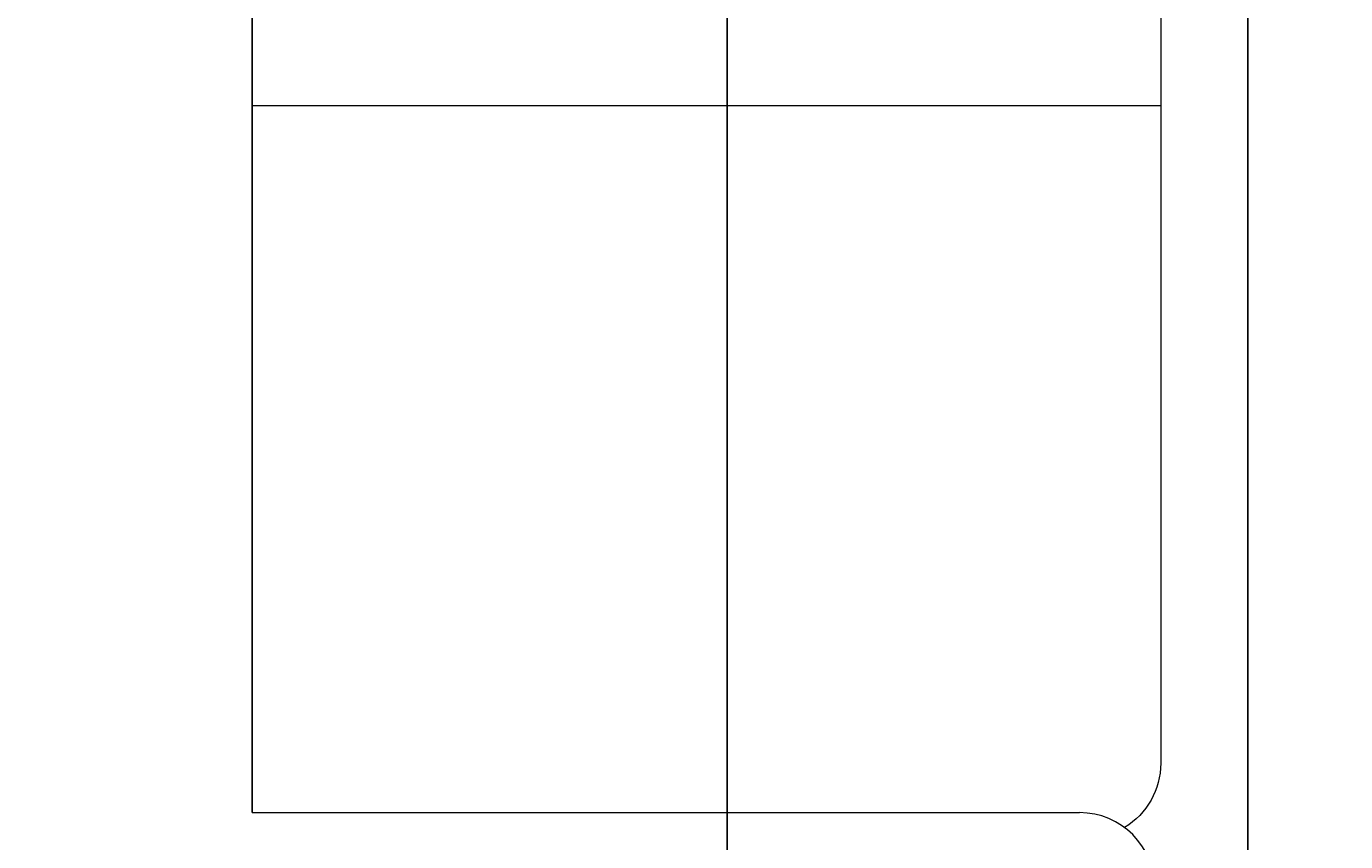
# Model space of a CAD drawing. Units: inches. Extents: x 2231 to 2461, y 2045 to 2455.
# Tile 39 of 95: x 2262 to 2297, y 2200 to 2222. Entities that reach past the tile are written whole.
import ezdxf

# ---------------------------------------------------------------- set-up
doc = ezdxf.new("R2010")
doc.units = ezdxf.units.IN
doc.layers.add('A-ANNO-DIMS', color=2, linetype='Continuous', lineweight=18)
doc.layers.add('A-FURN', color=9, linetype='Continuous', lineweight=18)
doc.styles.get("Standard").update_dxf_attribs({"font": 'arial.ttf'})
doc.dimstyles.get("Standard").update_dxf_attribs({"dimtxt": 0.18, "dimasz": 0.18, "dimexe": 0.18, "dimexo": 0.0625, "dimgap": 0.09, "dimtad": 0, "dimtih": 1, "dimtoh": 1, "dimdec": 4, "dimzin": 0, "dimdsep": 46, "dimtxsty": 'Standard', "dimcen": 0.09, "dimadec": 0, "dimazin": 0, "dimtfac": 1, "dimtdec": 4, "dimtofl": 0, "dimtmove": 0, "dimatfit": 3, "dimfxl": 1, "dimtolj": 1, "dimtzin": 0, "dimarcsym": 0})

# ---------------------------------------------------------------- blocks, each defined once
blk = doc.blocks.new('*D47')
at = {"layer": 'A-ANNO-DIMS', "color": 0, "lineweight": -2, "transparency": 16777216}
for p, q in [((2258.794, 2182.895), (2258.794, 2454.645)), ((2258.974, 2454.465), (2276.575, 2454.465)), ((2294.614, 2454.465), (2277.012, 2454.465)), ((2294.794, 2182.895), (2294.794, 2454.645))]:
    blk.add_line(p, q, dxfattribs=at)
at = {"layer": 'A-ANNO-DIMS', "color": 0, "transparency": 16777216}
for points in [[(2258.974, 2454.495), (2258.974, 2454.435), (2258.794, 2454.465)], [(2294.614, 2454.495), (2294.614, 2454.435), (2294.794, 2454.465)]]:
    blk.add_solid(points, dxfattribs=at)
at = {"layer": 'Defpoints', "color": 0, "transparency": 16777216}
for p in [(2294.794, 2454.465), (2258.794, 2182.833), (2294.794, 2182.833)]:
    blk.add_point(p, dxfattribs=at)
at = {"layer": 'A-ANNO-DIMS', "color": 0, "transparency": 16777216, "insert": (2276.794, 2454.465), "char_height": 0.18, "attachment_point": 5}
blk.add_mtext('\\A1;36', dxfattribs=at)
blk = doc.blocks.new('*D51')
at = {"layer": 'A-ANNO-DIMS', "color": 0, "lineweight": -2, "transparency": 16777216}
for p, q in [((2258.794, 2306.77), (2258.794, 2044.803)), ((2330.794, 2306.77), (2330.794, 2044.803)), ((2258.974, 2044.983), (2294.576, 2044.983)), ((2330.614, 2044.983), (2295.011, 2044.983))]:
    blk.add_line(p, q, dxfattribs=at)
at = {"layer": 'A-ANNO-DIMS', "color": 0, "transparency": 16777216}
for points in [[(2258.974, 2045.013), (2258.974, 2044.953), (2258.794, 2044.983)], [(2330.614, 2045.013), (2330.614, 2044.953), (2330.794, 2044.983)]]:
    blk.add_solid(points, dxfattribs=at)
at = {"layer": 'Defpoints', "color": 0, "transparency": 16777216}
for p in [(2258.794, 2306.833), (2330.794, 2306.833), (2330.794, 2044.983)]:
    blk.add_point(p, dxfattribs=at)
at = {"layer": 'A-ANNO-DIMS', "color": 0, "transparency": 16777216, "insert": (2294.794, 2044.983), "char_height": 0.18, "attachment_point": 5}
blk.add_mtext('\\A1;72', dxfattribs=at)
blk = doc.blocks.new('*D63')
at = {"layer": 'A-ANNO-DIMS', "color": 0, "lineweight": -2, "transparency": 16777216}
for p, q in [((2262.383, 2255.114), (2281.133, 2255.114)), ((2280.953, 2254.934), (2280.953, 2225.296)), ((2280.953, 2195.294), (2280.953, 2224.932)), ((2262.383, 2195.114), (2281.133, 2195.114))]:
    blk.add_line(p, q, dxfattribs=at)
at = {"layer": 'A-ANNO-DIMS', "color": 0, "transparency": 16777216}
for points in [[(2280.923, 2254.934), (2280.983, 2254.934), (2280.953, 2255.114)], [(2280.923, 2195.294), (2280.983, 2195.294), (2280.953, 2195.114)]]:
    blk.add_solid(points, dxfattribs=at)
at = {"layer": 'Defpoints', "color": 0, "transparency": 16777216}
for p in [(2262.321, 2255.114), (2262.321, 2195.114), (2280.953, 2195.114)]:
    blk.add_point(p, dxfattribs=at)
at = {"layer": 'A-ANNO-DIMS', "color": 0, "transparency": 16777216, "insert": (2280.953, 2225.114), "char_height": 0.18, "attachment_point": 5}
blk.add_mtext('\\A1;60', dxfattribs=at)

msp = doc.modelspace()

# ---------------------------------------------------------------- linework, layer by layer
at = {"layer": 'A-FURN'}
for p, q in [((2268.3207, 2249.1137), (2268.3207, 2201.1137)), ((2268.3207, 2201.1137), (2290.3207, 2201.1137))]:
    msp.add_line(p, q, dxfattribs=at)
for points in [[(2268.3207, 2210.1618), (2268.3207, 2229.6377)], [(2292.4784, 2229.6377), (2292.4784, 2210.1618)]]:
    msp.add_lwpolyline(points, dxfattribs=at)
msp.add_lwpolyline([(2268.3207, 2201.1137), (2268.3207, 2219.8998), (2292.4784, 2219.8998), (2292.4784, 2202.4238, -0.2617418), (2291.5184, 2200.7154, -0.2617418)], format="xyb", dxfattribs=at)
msp.add_arc((2290.3207, 2199.1137), 2, 0, 90, dxfattribs=at)

# ---------------------------------------------------------------- dimensions: what is measured, and where the dimension line sits
at = {"layer": 'A-ANNO-DIMS'}
for base, p1, p2, picture, middle in [((2294.7935, 2454.4653), (2258.7935, 2182.8328), (2294.7935, 2182.8328), '*D47', (2276.7935, 2454.4653)), ((2330.7935, 2044.9825), (2258.7935, 2306.8328), (2330.7935, 2306.8328), '*D51', (2294.7935, 2044.9825))]:
    dim = msp.add_linear_dim(base=base, p1=p1, p2=p2, dimstyle='Standard', override={"dimdec": 0, "dimlfac": 1, "dimrnd": 0, "dimzin": 0, "dimdsep": 46, "dimlunit": 2}, dxfattribs=at)
    dim.commit()
    dim.dimension.update_dxf_attribs({"geometry": picture, "text_midpoint": middle})
dim = msp.add_linear_dim(base=(2280.9532, 2195.1137), p1=(2262.3207, 2255.1137), p2=(2262.3207, 2195.1137), angle=270, dimstyle='Standard', override={"dimdec": 0, "dimlfac": 1, "dimrnd": 0, "dimzin": 0, "dimdsep": 46, "dimlunit": 2}, dxfattribs=at)
dim.commit()
dim.dimension.update_dxf_attribs({"geometry": '*D63', "text_midpoint": (2280.9532, 2225.1137)})

doc.saveas('drawing.dxf')
